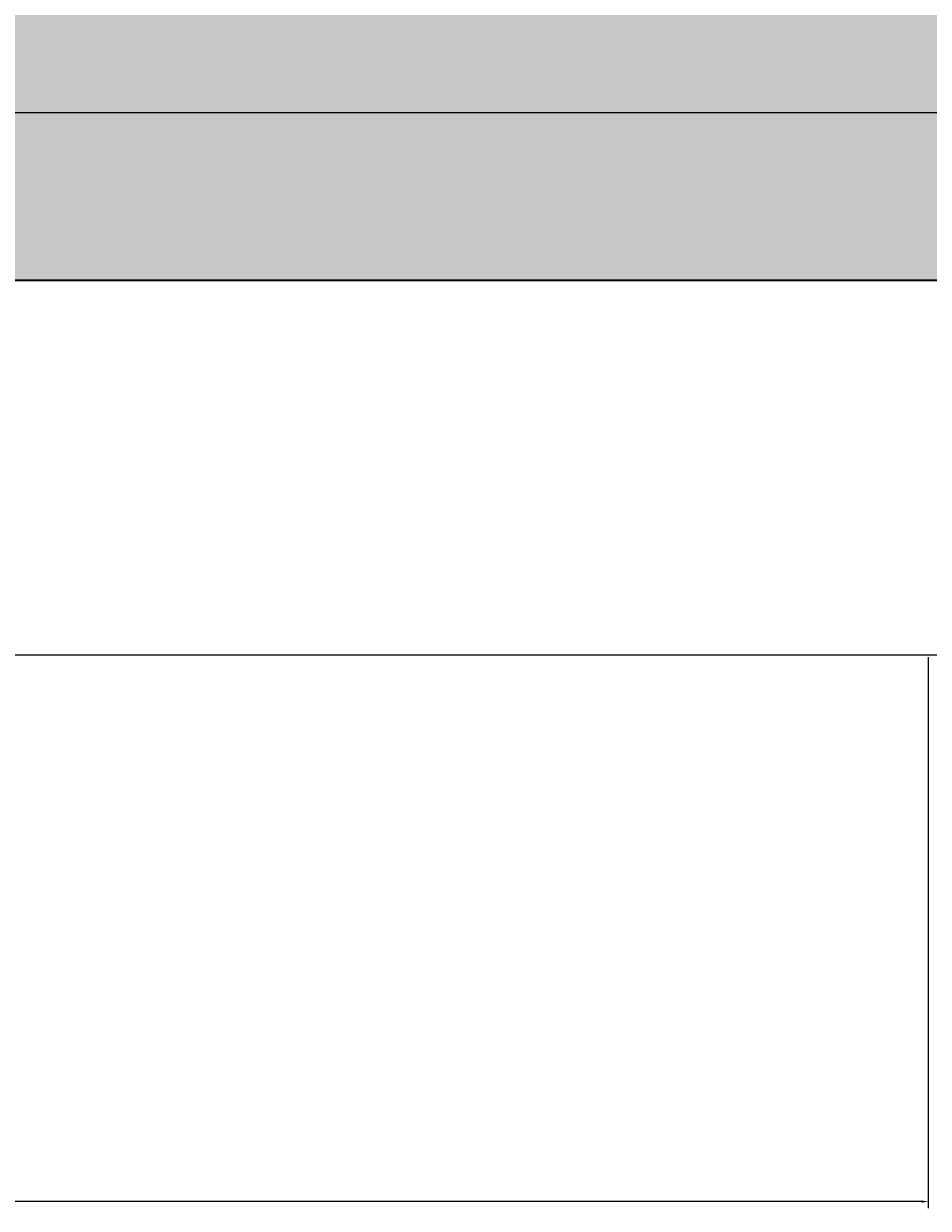
# Model space of a CAD drawing. Units: inches. Extents: x -1 to 292, y -3 to 199.
# Tile 17 of 52: x 124 to 148, y 11 to 42. Entities that reach past the tile are written whole.
import ezdxf

# ---------------------------------------------------------------- set-up
doc = ezdxf.new("R2010")
doc.units = ezdxf.units.IN
doc.header["$MEASUREMENT"] = 0
for name, color, linetype, lineweight in [('M-DIMS', 2, 'Continuous', 18), ('M-EQPM', 7, 'Continuous', 35), ('M-PATT', 8, 'Continuous', 13)]:
    doc.layers.add(name, color=color, linetype=linetype, lineweight=lineweight)
doc.styles.get("Standard").update_dxf_attribs({"font": 'arial.ttf'})
doc.dimstyles.get("Standard").update_dxf_attribs({"dimtxt": 0.18, "dimasz": 0.18, "dimexe": 0.18, "dimexo": 0.0625, "dimgap": 0.09, "dimtad": 0, "dimtih": 1, "dimtoh": 1, "dimdec": 4, "dimzin": 0, "dimdsep": 46, "dimtxsty": 'Standard', "dimcen": 0.09, "dimadec": 0, "dimazin": 0, "dimtfac": 1, "dimtdec": 4, "dimtofl": 0, "dimtmove": 0, "dimatfit": 3, "dimfxl": 1, "dimtolj": 1, "dimtzin": 0, "dimarcsym": 0})

# ---------------------------------------------------------------- blocks, each defined once
blk = doc.blocks.new('*D7')
at = {"layer": 'Defpoints', "color": 0, "transparency": 16777216}
for p in [(21.861, 54.582), (205.115, 54.582), (21.861, 39.982)]:
    blk.add_point(p, dxfattribs=at)
at = {"layer": 'M-DIMS', "color": 0, "lineweight": -2, "transparency": 16777216}
for p, q in [((21.861, 54.52), (21.861, 39.802)), ((205.115, 54.52), (205.115, 39.802)), ((22.041, 39.982), (113.033, 39.982)), ((204.935, 39.982), (113.944, 39.982))]:
    blk.add_line(p, q, dxfattribs=at)
at = {"layer": 'M-DIMS', "color": 0, "transparency": 16777216}
for points in [[(22.041, 40.012), (22.041, 39.952), (21.861, 39.982)], [(204.935, 40.012), (204.935, 39.952), (205.115, 39.982)]]:
    blk.add_solid(points, dxfattribs=at)
at = {"layer": 'M-DIMS', "color": 0, "transparency": 16777216, "insert": (113.488, 39.982), "char_height": 0.18, "attachment_point": 5}
blk.add_mtext('\\A1;183.25', dxfattribs=at)
blk = doc.blocks.new('*D11')
at = {"layer": 'Defpoints', "color": 0, "transparency": 16777216}
for p in [(79.013, 35.514), (292.04, 35.514), (79.013, 25.514)]:
    blk.add_point(p, dxfattribs=at)
at = {"layer": 'M-DIMS', "color": 0, "lineweight": -2, "transparency": 16777216}
for p, q in [((79.076, 35.514), (292.22, 35.514)), ((292.04, 35.334), (292.04, 30.696)), ((292.04, 25.694), (292.04, 30.332)), ((79.076, 25.514), (292.22, 25.514))]:
    blk.add_line(p, q, dxfattribs=at)
at = {"layer": 'M-DIMS', "color": 0, "transparency": 16777216}
for points in [[(292.01, 35.334), (292.07, 35.334), (292.04, 35.514)], [(292.01, 25.694), (292.07, 25.694), (292.04, 25.514)]]:
    blk.add_solid(points, dxfattribs=at)
at = {"layer": 'M-DIMS', "color": 0, "transparency": 16777216, "insert": (292.04, 30.514), "char_height": 0.18, "attachment_point": 5}
blk.add_mtext('\\A1;10', dxfattribs=at)
blk = doc.blocks.new('*D13')
at = {"layer": 'Defpoints', "color": 0, "transparency": 16777216}
for p in [(79.013, 25.514), (148.429, 25.514), (79.013, 10.914)]:
    blk.add_point(p, dxfattribs=at)
at = {"layer": 'M-DIMS', "color": 0, "lineweight": -2, "transparency": 16777216}
for p, q in [((79.013, 25.452), (79.013, 10.734)), ((148.429, 25.452), (148.429, 10.734)), ((79.193, 10.914), (113.328, 10.914)), ((148.249, 10.914), (114.115, 10.914))]:
    blk.add_line(p, q, dxfattribs=at)
at = {"layer": 'M-DIMS', "color": 0, "transparency": 16777216}
for points in [[(79.193, 10.944), (79.193, 10.884), (79.013, 10.914)], [(148.249, 10.944), (148.249, 10.884), (148.429, 10.914)]]:
    blk.add_solid(points, dxfattribs=at)
at = {"layer": 'M-DIMS', "color": 0, "transparency": 16777216, "insert": (113.721, 10.914), "char_height": 0.18, "attachment_point": 5}
blk.add_mtext('\\A1;69.42', dxfattribs=at)

msp = doc.modelspace()

# ---------------------------------------------------------------- hatches: boundary and pattern name
at = {"layer": 'M-PATT'}
h = msp.add_hatch(color=256, dxfattribs=at)
h.set_gradient(color1=(0, 255, 255), color2=(0, 255, 255), tint=1)
h.paths.add_polyline_path([(75.3521, 99.7735), (72.66, 101.3278), (70.2665, 99.7735), (67.5744, 101.3278), (65.1809, 99.7735), (62.4888, 101.3278), (60.0953, 99.7735), (57.4032, 101.3278), (55.0097, 99.7735), (52.3176, 101.3278), (49.9241, 99.7735, 0.4142136), (57.8007, 91.897), (61.6788, 91.897), (61.6788, 51.2672), (57.8007, 51.2672, 0.8088808), (54.5813, 36.2021), (65.0947, 51.2672), (64.6788, 51.2672), (64.6788, 91.897), (67.6788, 91.897), (67.6788, 51.2672), (65.0947, 51.2672), (54.5813, 36.2021, 0.1056561), (57.8007, 35.5141), (169.176, 35.5141, 1), (169.176, 51.2672), (162.6788, 51.2672), (162.6788, 91.897), (169.176, 91.897, 0.4144629), (177.0526, 99.7802), (174.372, 101.3278), (171.9786, 99.7735), (169.2864, 101.3278), (166.893, 99.7735), (164.2008, 101.3278), (162.1623, 100.004), (162.1623, 96.1027), (160.6222, 96.1027), (160.6222, 100.4578), (159.1152, 101.3278), (156.7218, 99.7735), (154.0296, 101.3278), (151.6362, 99.7735), (148.944, 101.3278), (146.5506, 99.7735), (143.8584, 101.3278), (141.465, 99.7735), (138.7728, 101.3278), (136.3794, 99.7735), (133.6872, 101.3278), (131.2938, 99.7735), (128.6016, 101.3278), (126.2082, 99.7735), (123.516, 101.3278), (121.1225, 99.7735), (118.4304, 101.3278), (116.0369, 99.7735), (113.3448, 101.3278), (110.9513, 99.7735), (108.2592, 101.3278), (105.8657, 99.7735), (103.1736, 101.3278), (100.7801, 99.7735), (98.088, 101.3278), (95.6945, 99.7735), (93.0024, 101.3278), (90.6089, 99.7735), (87.9168, 101.3278), (85.5233, 99.7735), (82.8312, 101.3278), (80.4377, 99.7735), (77.7456, 101.3278)])
h.paths.add_polyline_path([(79.6788, 91.897), (79.6788, 51.2672), (76.6788, 51.2672), (76.6788, 91.897)], flags=16)
h.paths.add_polyline_path([(73.6788, 91.897), (73.6788, 51.2672), (70.6788, 51.2672), (70.6788, 91.897)], flags=16)
h.paths.add_polyline_path([(82.6788, 91.897), (101.6788, 91.897), (101.6788, 51.2672), (82.6788, 51.2672)], flags=16)
h.paths.add_polyline_path([(104.6788, 91.897), (107.6788, 91.897), (107.6788, 51.2672), (104.6788, 51.2672)], flags=16)
h.paths.add_polyline_path([(110.6788, 91.897), (113.6788, 91.897), (113.6788, 51.2672), (110.6788, 51.2672)], flags=16)
h.paths.add_polyline_path([(116.6788, 91.897), (119.6788, 91.897), (119.6788, 51.2672), (116.6788, 51.2672)], flags=16)
h.paths.add_polyline_path([(122.6788, 91.897), (141.6788, 91.897), (141.6788, 51.2672), (144.6788, 51.2672), (144.6788, 91.897), (147.6788, 91.897), (147.6788, 51.2672), (122.6788, 51.2672)], flags=16)
h.paths.add_polyline_path([(150.6788, 91.897), (153.6788, 91.897), (153.6788, 51.2672), (150.6788, 51.2672)], flags=16)
h.paths.add_polyline_path([(156.6788, 91.897), (159.6788, 91.897), (159.6788, 51.2672), (156.6788, 51.2672)], flags=16)

# ---------------------------------------------------------------- linework, layer by layer
at = {"layer": 'M-EQPM'}
msp.add_lwpolyline([(61.6788, 51.2672), (57.8007, 51.2672, 1), (57.8007, 35.5141), (169.176, 35.5141, 1), (169.176, 51.2672), (162.6788, 51.2672)], format="xyb", dxfattribs=at)

# ---------------------------------------------------------------- dimensions: what is measured, and where the dimension line sits
at = {"layer": 'M-DIMS'}
for base, p1, p2, angle, override, picture, middle in [((21.8612, 39.9821), (205.1155, 54.5821), (21.8612, 54.5821), 180, {"dimdec": 2, "dimlfac": 1, "dimrnd": 0, "dimzin": 0, "dimdsep": 46, "dimlunit": 2}, '*D7', (113.4883, 39.9821)), ((292.0399, 35.5141), (79.013, 25.5141), (79.013, 35.5141), 90, {"dimdec": 0, "dimlfac": 1, "dimrnd": 0, "dimzin": 0, "dimdsep": 46, "dimlunit": 2}, '*D11', (292.0399, 30.5141)), ((79.013, 10.9141), (148.4295, 25.5141), (79.013, 25.5141), 180, {"dimdec": 2, "dimlfac": 1, "dimrnd": 0, "dimzin": 0, "dimdsep": 46, "dimlunit": 2}, '*D13', (113.7212, 10.9141))]:
    dim = msp.add_linear_dim(base=base, p1=p1, p2=p2, angle=angle, dimstyle='Standard', override=override, dxfattribs=at)
    dim.commit()
    dim.dimension.update_dxf_attribs({"geometry": picture, "text_midpoint": middle})

doc.saveas('drawing.dxf')
